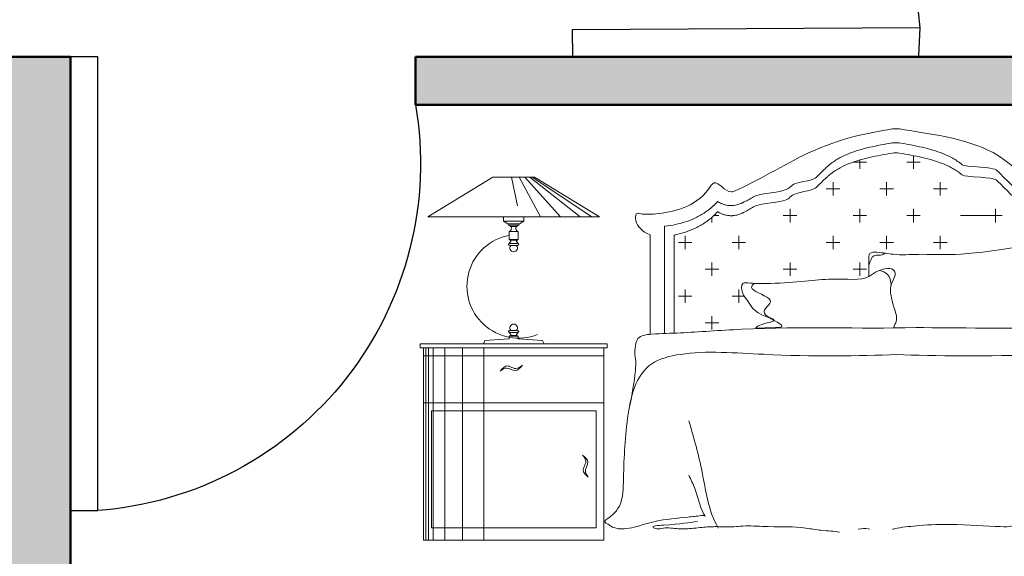
# Model space of a CAD drawing. Units: inches. Extents: x 1771 to 3025, y 319 to 889.
# Tile 16 of 35: x 2402 to 2505, y 564 to 621. Entities that reach past the tile are written whole.
import ezdxf

# ---------------------------------------------------------------- set-up
doc = ezdxf.new("R2010")
doc.units = ezdxf.units.IN
doc.header["$MEASUREMENT"] = 0
for name, color, linetype, lineweight in [('A-DOOR', 4, 'Continuous', 25), ('A-FURN', 8, 'Continuous', 18), ('A-WALL', 7, 'Continuous', 50), ('A-WALL-PATT', 254, 'Continuous', 13)]:
    doc.layers.add(name, color=color, linetype=linetype, lineweight=lineweight)

# ---------------------------------------------------------------- blocks, each defined once
blk = doc.blocks.new('A$C3908634B')
at = {"ltscale": 5}
for p, q in [((1200.2, 1046.3), (1218.1, 1046.3)), ((1176, 731), (1176, 731.7))]:
    blk.add_line(p, q, dxfattribs=at)
for p, q in [((1253.9, 945.1), (1253.9, 978.5)), ((1100.9, 962.2), (1134.6, 962.2)), ((1117.6, 945.1), (1117.6, 967.5)), ((1236.9, 962.2), (1271, 962.2)), ((184.3, 923.4), (19, 823.1)), ((237.5, 923.4), (184.3, 923.4)), ((190.2, 923.4), (237.5, 923.4)), ((231.9, 923.4), (247.3, 851.1)), ((284.7, 923.4), (237.5, 923.4)), ((237.5, 923.4), (290.6, 923.4)), ((251.7, 923.4), (305.7, 823.1)), ((266, 923.4), (356.4, 823.1)), ((278.7, 923.4), (406.8, 823.1)), ((284.7, 923.4), (436.3, 823.1)), ((290.6, 923.4), (456, 823.1)), ((1049.4, 876.9), (1049.4, 911)), ((1185.7, 876.9), (1185.7, 911)), ((1322.1, 876.9), (1322.1, 911)), ((2198.9, 923.4), (2033.5, 823.1)), ((2204.8, 923.4), (2053.3, 823.1)), ((2210.8, 923.4), (2082.7, 823.1)), ((2223.5, 923.4), (2133.1, 823.1)), ((2237.8, 923.4), (2183.8, 823.1)), ((2252, 923.4), (2198.9, 923.4)), ((2204.8, 923.4), (2252, 923.4)), ((2257.6, 923.4), (2242.2, 851.1)), ((2299.3, 923.4), (2252, 923.4)), ((2252, 923.4), (2305.2, 923.4)), ((2305.2, 923.4), (2470.5, 823.1)), ((1032.3, 894), (1066.4, 894)), ((1168.7, 894), (1202.8, 894)), ((1305.1, 894), (1339.1, 894)), ((940, 808.8), (940, 842.9)), ((1117.6, 808.8), (1117.6, 842.9)), ((1253.9, 808.8), (1253.9, 842.9)), ((1462.5, 808.8), (1462.5, 842.9)), ((237.5, 823.1), (19, 823.1)), ((212, 823.1), (212, 811.7)), ((212, 811.7), (223, 805.4)), ((212, 811.7), (237.5, 811.7)), ((223, 805.4), (224.6, 801.4)), ((223, 805.4), (237.5, 805.4)), ((250.4, 801.4), (224.6, 801.4)), ((226.9, 801.4), (228.3, 798.3)), ((237.5, 823.1), (456, 823.1)), ((263, 811.7), (237.5, 811.7)), ((252, 805.4), (237.5, 805.4)), ((248.1, 801.4), (246.7, 798.3)), ((252, 805.4), (250.4, 801.4)), ((263, 811.7), (252, 805.4)), ((263, 823.1), (263, 811.7)), ((741.7, 808.8), (741.7, 821.7)), ((746.2, 825.8), (758.8, 825.8)), ((922.9, 825.8), (957, 825.8)), ((1100.5, 825.8), (1134.6, 825.8)), ((1236.9, 825.8), (1271, 825.8)), ((1373.2, 825.8), (1479.5, 825.8)), ((1681.3, 808.8), (1681.3, 825.6)), ((2252, 823.1), (2033.5, 823.1)), ((2226.5, 823.1), (2226.5, 811.7)), ((2226.5, 811.7), (2237.6, 805.4)), ((2226.5, 811.7), (2252, 811.7)), ((2237.6, 805.4), (2239.1, 801.4)), ((2237.6, 805.4), (2252, 805.4)), ((2239.1, 801.4), (2264.9, 801.4)), ((2241.4, 801.4), (2242.8, 798.3)), ((2252, 823.1), (2470.5, 823.1)), ((2277.6, 811.7), (2252, 811.7)), ((2266.5, 805.4), (2252, 805.4)), ((2262.6, 801.4), (2261.2, 798.3)), ((2266.5, 805.4), (2264.9, 801.4)), ((2277.6, 811.7), (2266.5, 805.4)), ((2277.6, 823.1), (2277.6, 811.7)), ((227.8, 786.4), (226.2, 785.6)), ((226.2, 785.6), (226.2, 765)), ((226.2, 785.6), (248.8, 785.6)), ((230.2, 788), (227.8, 786.4)), ((228.3, 798.3), (237.5, 798.3)), ((228.3, 798.3), (231.3, 797.6)), ((231.1, 790.5), (230.2, 788)), ((231.5, 791.1), (231.1, 790.5)), ((231.3, 797.6), (232, 794.9)), ((231.6, 792.6), (231.5, 791.9)), ((231.5, 791.9), (231.5, 791.1)), ((231.9, 793.9), (231.6, 792.6)), ((232, 794.9), (231.9, 793.9)), ((246.7, 798.3), (237.5, 798.3)), ((243.7, 797.6), (243, 794.9)), ((243, 794.9), (243.1, 793.9)), ((243.1, 793.9), (243.4, 792.6)), ((243.4, 792.6), (243.4, 791.9)), ((243.4, 791.9), (243.4, 791.1)), ((243.4, 791.1), (243.9, 790.5)), ((246.7, 798.3), (243.7, 797.6)), ((243.9, 790.5), (244.8, 788)), ((244.8, 788), (247.2, 786.4)), ((247.2, 786.4), (248.8, 785.6)), ((248.8, 785.6), (248.8, 765)), ((621.3, 798.8), (621.3, 526)), ((645.8, 776.5), (645.8, 527)), ((1824, 776.5), (1824, 527.2)), ((1848.6, 798.8), (1848.6, 526.2)), ((2242.3, 786.4), (2240.7, 785.6)), ((2240.7, 785.6), (2240.7, 765)), ((2263.3, 785.6), (2240.7, 785.6)), ((2244.7, 788), (2242.3, 786.4)), ((2242.8, 798.3), (2245.8, 797.6)), ((2242.8, 798.3), (2252, 798.3)), ((2245.6, 790.5), (2244.7, 788)), ((2246.1, 791.1), (2245.6, 790.5)), ((2245.8, 797.6), (2246.5, 794.9)), ((2246.4, 793.9), (2246.1, 792.6)), ((2246.1, 792.6), (2246.1, 791.9)), ((2246.1, 791.9), (2246.1, 791.1)), ((2246.5, 794.9), (2246.4, 793.9)), ((2261.2, 798.3), (2252, 798.3)), ((2258.2, 797.6), (2257.6, 794.9)), ((2257.6, 794.9), (2257.6, 793.9)), ((2257.6, 793.9), (2257.9, 792.6)), ((2257.9, 792.6), (2258, 791.9)), ((2258, 791.9), (2258, 791.1)), ((2258, 791.1), (2258.4, 790.5)), ((2261.2, 798.3), (2258.2, 797.6)), ((2258.4, 790.5), (2259.4, 788)), ((2259.4, 788), (2261.7, 786.4)), ((2261.7, 786.4), (2263.3, 785.6)), ((2263.3, 785.6), (2263.3, 765)), ((224.8, 753.5), (224.7, 752.9)), ((224.7, 752.9), (224.8, 752.1)), ((225.3, 753.9), (224.8, 753.5)), ((224.8, 752.1), (225.2, 751.4)), ((225.2, 751.4), (225.6, 750.9)), ((225.7, 754.3), (225.3, 753.9)), ((225.6, 750.9), (228.1, 750.2)), ((226.3, 754.6), (225.7, 754.3)), ((226.2, 765), (227.6, 764.2)), ((226.2, 765), (237.5, 765)), ((227, 754.7), (226.3, 754.6)), ((227.9, 754.7), (227, 754.7)), ((227.4, 757.9), (227.1, 757.2)), ((227.1, 757.2), (227.3, 756.6)), ((227.3, 756.6), (227.8, 755.9)), ((227.7, 758.5), (227.4, 757.9)), ((227.6, 764.2), (228.5, 763.3)), ((228.6, 758.7), (227.7, 758.5)), ((227.8, 755.9), (228.9, 755.2)), ((228.9, 755.2), (227.9, 754.7)), ((228.5, 763.3), (229.4, 762.5)), ((228.5, 763.3), (237.5, 763.3)), ((229.4, 759.1), (228.6, 758.7)), ((228.9, 755.2), (237.5, 755.2)), ((229.4, 762.5), (230, 761.4)), ((229.8, 759.5), (229.4, 759.1)), ((230.1, 760.2), (229.8, 759.5)), ((230, 761.4), (230.1, 760.2)), ((248.8, 765), (237.5, 765)), ((246.5, 763.3), (237.5, 763.3)), ((246.1, 755.2), (237.5, 755.2)), ((245, 761.4), (244.9, 760.2)), ((244.9, 760.2), (245.2, 759.5)), ((245.6, 762.5), (245, 761.4)), ((245.2, 759.5), (245.6, 759.1)), ((246.5, 763.3), (245.6, 762.5)), ((245.6, 759.1), (246.4, 758.7)), ((247.2, 755.9), (246.1, 755.2)), ((246.1, 755.2), (247.1, 754.7)), ((246.4, 758.7), (247.3, 758.5)), ((247.4, 764.2), (246.5, 763.3)), ((249.4, 750.9), (246.9, 750.2)), ((247.1, 754.7), (248, 754.7)), ((247.7, 756.6), (247.2, 755.9)), ((247.3, 758.5), (247.6, 757.9)), ((248.8, 765), (247.4, 764.2)), ((247.6, 757.9), (247.9, 757.2)), ((247.9, 757.2), (247.7, 756.6)), ((248, 754.7), (248.7, 754.6)), ((248.7, 754.6), (249.3, 754.3)), ((249.3, 754.3), (249.7, 753.9)), ((249.8, 751.4), (249.4, 750.9)), ((249.7, 753.9), (250.2, 753.5)), ((250.2, 752.1), (249.8, 751.4)), ((250.2, 753.5), (250.3, 752.9)), ((250.3, 752.9), (250.2, 752.1)), ((656.5, 757.6), (690.6, 757.6)), ((673.5, 740.6), (673.5, 774.7)), ((792.9, 757.6), (827, 757.6)), ((809.9, 740.6), (809.9, 774.7)), ((1032.3, 757.6), (1066.4, 757.6)), ((1049.4, 740.6), (1049.4, 774.7)), ((1168.7, 757.6), (1202.8, 757.6)), ((1185.7, 740.6), (1185.7, 774.7)), ((1305.1, 757.6), (1339.1, 757.6)), ((1322.1, 740.6), (1322.1, 774.7)), ((1513.6, 757.6), (1547.7, 757.6)), ((1530.6, 751.3), (1530.6, 774.7)), ((1732.4, 757.6), (1766.5, 757.6)), ((1749.5, 740.6), (1749.5, 774.7)), ((2239.4, 753.5), (2239.2, 752.9)), ((2239.2, 752.9), (2239.3, 752.1)), ((2239.3, 752.1), (2239.7, 751.4)), ((2239.9, 753.9), (2239.4, 753.5)), ((2239.7, 751.4), (2240.2, 750.9)), ((2240.3, 754.3), (2239.9, 753.9)), ((2240.2, 750.9), (2242.6, 750.2)), ((2240.8, 754.6), (2240.3, 754.3)), ((2240.7, 765), (2242.1, 764.2)), ((2240.7, 765), (2252, 765)), ((2241.5, 754.7), (2240.8, 754.6)), ((2242.4, 754.7), (2241.5, 754.7)), ((2241.9, 757.9), (2241.7, 757.2)), ((2241.7, 757.2), (2241.8, 756.6)), ((2241.8, 756.6), (2242.3, 755.9)), ((2242.2, 758.5), (2241.9, 757.9)), ((2242.1, 764.2), (2243, 763.3)), ((2243.1, 758.7), (2242.2, 758.5)), ((2242.3, 755.9), (2243.4, 755.2)), ((2243.4, 755.2), (2242.4, 754.7)), ((2243, 763.3), (2243.9, 762.5)), ((2243, 763.3), (2252, 763.3)), ((2243.9, 759.1), (2243.1, 758.7)), ((2243.4, 755.2), (2252, 755.2)), ((2243.9, 762.5), (2244.6, 761.4)), ((2244.3, 759.5), (2243.9, 759.1)), ((2244.6, 760.2), (2244.3, 759.5)), ((2244.6, 761.4), (2244.6, 760.2)), ((2263.3, 765), (2252, 765)), ((2261.1, 763.3), (2252, 763.3)), ((2260.7, 755.2), (2252, 755.2)), ((2259.5, 761.4), (2259.4, 760.2)), ((2259.4, 760.2), (2259.7, 759.5)), ((2260.1, 762.5), (2259.5, 761.4)), ((2259.7, 759.5), (2260.1, 759.1)), ((2261.1, 763.3), (2260.1, 762.5)), ((2260.1, 759.1), (2260.9, 758.7)), ((2261.8, 755.9), (2260.7, 755.2)), ((2260.7, 755.2), (2261.6, 754.7)), ((2260.9, 758.7), (2261.8, 758.5)), ((2261.9, 764.2), (2261.1, 763.3)), ((2263.9, 750.9), (2261.5, 750.2)), ((2261.6, 754.7), (2262.5, 754.7)), ((2261.8, 758.5), (2262.2, 757.9)), ((2262.2, 756.6), (2261.8, 755.9)), ((2263.3, 765), (2261.9, 764.2)), ((2262.2, 757.9), (2262.4, 757.2)), ((2262.4, 757.2), (2262.2, 756.6)), ((2262.5, 754.7), (2263.2, 754.6)), ((2263.2, 754.6), (2263.8, 754.3)), ((2263.8, 754.3), (2264.2, 753.9)), ((2264.3, 751.4), (2263.9, 750.9)), ((2264.2, 753.9), (2264.7, 753.5)), ((2264.7, 752.1), (2264.3, 751.4)), ((2264.7, 753.5), (2264.8, 752.9)), ((2264.8, 752.9), (2264.7, 752.1)), ((228.1, 750.2), (229.9, 750)), ((229.9, 750), (232.4, 750.2)), ((232.4, 750.2), (237.5, 750.2)), ((242.6, 750.2), (237.5, 750.2)), ((245.1, 750), (242.6, 750.2)), ((246.9, 750.2), (245.1, 750)), ((2242.6, 750.2), (2244.4, 750)), ((2244.4, 750), (2246.9, 750.2)), ((2246.9, 750.2), (2252, 750.2)), ((2257.1, 750.2), (2252, 750.2)), ((2259.6, 750), (2257.1, 750.2)), ((2261.5, 750.2), (2259.6, 750)), ((741.7, 672.4), (741.7, 706.5)), ((940, 672.4), (940, 706.5)), ((1117.6, 672.4), (1117.6, 706.5)), ((1681.3, 672.4), (1681.3, 706.5)), ((1817.7, 672.4), (1817.7, 706.5)), ((724.7, 689.4), (758.8, 689.4)), ((922.9, 689.4), (957, 689.4)), ((1100.5, 689.4), (1134.6, 689.4)), ((1664.3, 689.4), (1698.3, 689.4)), ((1800.6, 689.4), (1824, 689.4)), ((673.5, 604.2), (673.5, 638.3)), ((809.9, 604.2), (809.9, 638.3)), ((1749.5, 604.2), (1749.5, 638.3)), ((656.5, 621.3), (690.6, 621.3)), ((792.9, 621.3), (823.2, 621.3)), ((1732.4, 621.3), (1766.5, 621.3)), ((724.7, 553.1), (758.8, 553.1)), ((741.7, 536), (741.7, 570.1)), ((1664.3, 553.1), (1698.3, 553.1)), ((1681.3, 536), (1681.3, 570.1)), ((1800.6, 553.1), (1824, 553.1)), ((1817.7, 536), (1817.7, 570.1)), ((224.7, 530.9), (224.8, 531.7)), ((224.8, 530.3), (224.7, 530.9)), ((224.8, 531.7), (225.2, 532.4)), ((225.3, 529.9), (224.8, 530.3)), ((225.2, 532.4), (225.6, 532.9)), ((225.7, 529.5), (225.3, 529.9)), ((225.6, 532.9), (228.1, 533.6)), ((226.3, 529.2), (225.7, 529.5)), ((227, 529.1), (226.3, 529.2)), ((227.9, 529.1), (227, 529.1)), ((227.1, 526.6), (227.3, 527.2)), ((227.4, 525.9), (227.1, 526.6)), ((227.3, 527.2), (227.8, 527.9)), ((227.7, 525.3), (227.4, 525.9)), ((227.8, 527.9), (228.9, 528.6)), ((228.9, 528.6), (227.9, 529.1)), ((228.1, 533.6), (229.9, 533.8)), ((228.9, 528.6), (237.5, 528.6)), ((230.3, 533.8), (237.5, 533.6)), ((242.6, 533.6), (237.5, 533.6)), ((246.1, 528.6), (237.5, 528.6)), ((245.1, 533.8), (242.6, 533.6)), ((246.9, 533.6), (245.1, 533.8)), ((246.1, 528.6), (247.1, 529.1)), ((247.2, 527.9), (246.1, 528.6)), ((249.4, 532.9), (246.9, 533.6)), ((247.1, 529.1), (248, 529.1)), ((247.7, 527.2), (247.2, 527.9)), ((247.3, 525.3), (247.6, 525.9)), ((247.6, 525.9), (247.9, 526.6)), ((247.9, 526.6), (247.7, 527.2)), ((248, 529.1), (248.7, 529.2)), ((248.7, 529.2), (249.3, 529.5)), ((249.3, 529.5), (249.7, 529.9)), ((249.8, 532.4), (249.4, 532.9)), ((249.7, 529.9), (250.2, 530.3)), ((250.2, 531.7), (249.8, 532.4)), ((250.3, 530.9), (250.2, 531.7)), ((250.2, 530.3), (250.3, 530.9)), ((2239.2, 530.9), (2239.3, 531.7)), ((2239.4, 530.3), (2239.2, 530.9)), ((2239.3, 531.7), (2239.7, 532.4)), ((2239.9, 529.9), (2239.4, 530.3)), ((2239.7, 532.4), (2240.2, 532.9)), ((2240.3, 529.5), (2239.9, 529.9)), ((2240.2, 532.9), (2242.6, 533.6)), ((2240.8, 529.2), (2240.3, 529.5)), ((2241.5, 529.1), (2240.8, 529.2)), ((2242.4, 529.1), (2241.5, 529.1)), ((2241.7, 526.6), (2241.8, 527.2)), ((2241.9, 525.9), (2241.7, 526.6)), ((2241.8, 527.2), (2242.3, 527.9)), ((2242.2, 525.3), (2241.9, 525.9)), ((2242.3, 527.9), (2243.4, 528.6)), ((2243.4, 528.6), (2242.4, 529.1)), ((2242.6, 533.6), (2244.4, 533.8)), ((2243.4, 528.6), (2252, 528.6)), ((2244.4, 533.8), (2246.9, 533.6)), ((2246.9, 533.6), (2252, 533.6)), ((2259.2, 533.8), (2252, 533.6)), ((2260.7, 528.6), (2252, 528.6)), ((2261.5, 533.6), (2259.6, 533.8)), ((2260.7, 528.6), (2261.6, 529.1)), ((2261.8, 527.9), (2260.7, 528.6)), ((2263.9, 532.9), (2261.5, 533.6)), ((2261.6, 529.1), (2262.5, 529.1)), ((2262.2, 527.2), (2261.8, 527.9)), ((2261.8, 525.3), (2262.2, 525.9)), ((2262.4, 526.6), (2262.2, 527.2)), ((2262.2, 525.9), (2262.4, 526.6)), ((2262.5, 529.1), (2263.2, 529.2)), ((2263.2, 529.2), (2263.8, 529.5)), ((2263.8, 529.5), (2264.2, 529.9)), ((2264.3, 532.4), (2263.9, 532.9)), ((2264.2, 529.9), (2264.7, 530.3)), ((2264.7, 531.7), (2264.3, 532.4)), ((2264.8, 530.9), (2264.7, 531.7)), ((2264.7, 530.3), (2264.8, 530.9)), ((164, 507.9), (161.1, 499.5)), ((164, 507.9), (226.2, 512.1)), ((226.2, 518.8), (227.6, 519.6)), ((226.2, 512.1), (226.2, 518.8)), ((226.2, 518.8), (237.5, 518.8)), ((227.6, 519.6), (228.5, 520.5)), ((228.6, 525.1), (227.7, 525.3)), ((228.5, 520.5), (229.4, 521.3)), ((229.4, 524.7), (228.6, 525.1)), ((229.8, 524.3), (229.4, 524.7)), ((229.4, 521.3), (230, 522.4)), ((229.4, 521.3), (237.5, 521.3)), ((230.1, 523.6), (229.8, 524.3)), ((230, 522.4), (230.1, 523.6)), ((245.6, 521.3), (237.5, 521.3)), ((248.8, 518.8), (237.5, 518.8)), ((244.9, 523.6), (245.2, 524.3)), ((245, 522.4), (244.9, 523.6)), ((245.6, 521.3), (245, 522.4)), ((245.2, 524.3), (245.6, 524.7)), ((245.6, 524.7), (246.4, 525.1)), ((246.5, 520.5), (245.6, 521.3)), ((246.4, 525.1), (247.3, 525.3)), ((247.4, 519.6), (246.5, 520.5)), ((248.8, 518.8), (247.4, 519.6)), ((248.8, 512.1), (248.8, 518.8)), ((311, 507.9), (248.8, 512.1)), ((311, 507.9), (315.3, 499.5)), ((2178.5, 507.9), (2174.2, 499.5)), ((2178.5, 507.9), (2240.7, 512.1)), ((2240.7, 518.8), (2242.1, 519.6)), ((2240.7, 512.1), (2240.7, 518.8)), ((2240.7, 518.8), (2252, 518.8)), ((2242.1, 519.6), (2243, 520.5)), ((2243.1, 525.1), (2242.2, 525.3)), ((2243, 520.5), (2243.9, 521.3)), ((2243.9, 524.7), (2243.1, 525.1)), ((2244.3, 524.3), (2243.9, 524.7)), ((2243.9, 521.3), (2244.6, 522.4)), ((2243.9, 521.3), (2252, 521.3)), ((2244.6, 523.6), (2244.3, 524.3)), ((2244.6, 522.4), (2244.6, 523.6)), ((2260.1, 521.3), (2252, 521.3)), ((2263.3, 518.8), (2252, 518.8)), ((2259.4, 523.6), (2259.7, 524.3)), ((2259.5, 522.4), (2259.4, 523.6)), ((2260.1, 521.3), (2259.5, 522.4)), ((2259.7, 524.3), (2260.1, 524.7)), ((2260.1, 524.7), (2260.9, 525.1)), ((2261.1, 520.5), (2260.1, 521.3)), ((2260.9, 525.1), (2261.8, 525.3)), ((2261.9, 519.6), (2261.1, 520.5)), ((2263.3, 518.8), (2261.9, 519.6)), ((2263.3, 512.1), (2263.3, 518.8)), ((2325.5, 507.9), (2263.3, 512.1)), ((2325.5, 507.9), (2328.4, 499.5)), ((475, 499.5), (0, 499.5)), ((0, 499.5), (0, 489.5)), ((475, 489.5), (0, 489.5)), ((8.7, 489.5), (8.7, 0)), ((14.1, 488.6), (14.1, 0)), ((21.3, 488.6), (21.3, 0)), ((33, 488.6), (33, 0)), ((62.7, 488.6), (62.7, 0)), ((107.6, 488.6), (107.6, 0)), ((161.1, 499.5), (237.5, 499.5)), ((161.6, 488.6), (161.6, 0)), ((315.3, 499.5), (237.5, 499.5)), ((467.1, 0), (467.1, 489.5)), ((475, 499.5), (475, 489.5)), ((2014.5, 499.5), (2489.5, 499.5)), ((2014.5, 499.5), (2014.5, 489.5)), ((2014.5, 489.5), (2489.5, 489.5)), ((2022.4, 0), (2022.4, 489.5)), ((2174.2, 499.5), (2252, 499.5)), ((2328.4, 499.5), (2252, 499.5)), ((2327.9, 488.6), (2327.9, 0)), ((2381.9, 488.6), (2381.9, 0)), ((2426.8, 488.6), (2426.8, 0)), ((2456.5, 488.6), (2456.5, 0)), ((2468.2, 488.6), (2468.2, 0)), ((2475.4, 488.6), (2475.4, 0)), ((2480.8, 489.5), (2480.8, 0)), ((2489.5, 499.5), (2489.5, 489.5)), ((467.1, 469.5), (8.7, 469.5)), ((2022.4, 469.5), (2480.8, 469.5)), ((467.1, 349.5), (8.7, 349.5)), ((28.7, 329.5), (28.7, 31.6)), ((447.1, 329.5), (28.7, 329.5)), ((447.1, 31.6), (447.1, 329.5)), ((2022.4, 349.5), (2480.8, 349.5)), ((2042.4, 329.5), (2460.8, 329.5)), ((2042.4, 31.6), (2042.4, 329.5)), ((2460.8, 329.5), (2460.8, 31.6)), ((467.1, 281.6), (467.1, 301.6)), ((2022.4, 281.6), (2022.4, 301.6)), ((28.7, 31.6), (447.1, 31.6)), ((2460.8, 31.6), (2042.4, 31.6)), ((8.7, 0), (467.1, 0)), ((2022.4, 0), (2480.8, 0))]:
    blk.add_line(p, q)
at = {"ltscale": 20}
for p, q in [((584.4, 776.7), (584.4, 523.7)), ((1885.4, 776.7), (1885.4, 524))]:
    blk.add_line(p, q, dxfattribs=at)
for centre, radius, start, end in [((1209.1, 956.2), 55.2, 80.5605, 99.4395), ((1209.1, 930.3), 55.2, 80.5605, 99.4395), ((250.5, 646.2), 131.8, 100.6234, 291.2), ((2239, 646.2), 131.8, 248.8, 79.3766), ((237.5, 743.5), 9.69, 137.7341, 270), ((237.5, 743.5), 9.69, 270, 42.2659), ((2252, 743.5), 9.69, 137.7341, 270), ((2252, 743.5), 9.69, 270, 42.2659), ((237.5, 540.3), 9.69, 90, 222.2659), ((237.5, 540.3), 9.69, 317.7341, 90), ((2252, 540.3), 9.69, 90, 222.2659), ((2252, 540.3), 9.69, 317.7341, 90)]:
    blk.add_arc(centre, radius, start, end)
for points in [[(584.4, 776.7), (563.9, 786.2), (546, 802.1), (547.3, 834.8), (564.5, 828.3), (620.6, 830.4), (706.4, 847.2), (752.1, 924.2), (778.1, 880.4), (846.1, 907.1), (1017.7, 1014.1), (1134.5, 1035.5), (1200.2, 1046.3)], [(1885.4, 776.7), (1905.9, 786.2), (1923.9, 802.1), (1922.5, 834.8), (1905.3, 828.3), (1849.2, 830.4), (1763.4, 847.2), (1717.7, 924.2), (1691.7, 880.4), (1541.2, 907.1), (1472.8, 1014.1), (1283.8, 1035.5), (1218.1, 1046.3)]]:
    blk.add_open_spline(points, degree=3, knots=[12.417853, 12.417853, 12.417853, 12.417853, 68.394536, 90.665986, 114.156853, 157.554067, 281.869614, 298.858744, 338.737111, 347.060176, 470.423438, 625.498764, 625.498764, 625.498764, 625.498764], dxfattribs=at)
for points, knots in [([(756.1, 861.8), (756.9, 861.3), (757.6, 860.9), (759.9, 859.6), (761.6, 858.7), (765.5, 856.8), (767.8, 855.8), (772.7, 854.1), (775.4, 853.3), (780.8, 852.2), (783.3, 851.8), (787.1, 851.6), (788.2, 851.5), (789.9, 851.5), (790.6, 851.5), (791.9, 851.5), (792.5, 851.5), (793.6, 851.6), (794.1, 851.6), (795.8, 851.8), (796.8, 851.9), (800.3, 852.3), (802.5, 852.8), (806.5, 853.8), (808.3, 854.3), (811.5, 855.4), (812.9, 855.9), (815.3, 856.9), (816.4, 857.4), (817.6, 857.9), (817.8, 858), (818.4, 858.2), (818.7, 858.4), (819.5, 858.7), (820, 859), (821.6, 859.7), (822.7, 860.2), (825.8, 861.7), (827.9, 862.8), (834, 866), (837.9, 868.3), (848.5, 874.9), (854.9, 879.4), (928.8, 888.8), (934.4, 893.5), (945, 903.2), (950, 908), (1000.9, 917.4), (1005.5, 922.1), (1014.4, 931), (1018.7, 935.3), (1027, 943.5), (1031.1, 947.3), (1036.9, 952.4), (1038.8, 954), (1042, 956.7), (1043.5, 957.9), (1045.8, 959.7), (1046.7, 960.3), (1048.5, 961.7), (1049.4, 962.3), (1052.1, 964.2), (1054, 965.5), (1059.7, 969.2), (1063.6, 971.5), (1074.8, 977.5), (1082.2, 980.9), (1098, 987.2), (1106.3, 990), (1123.7, 995.2), (1132.8, 997.5), (1151.5, 1001.8), (1161.1, 1003.8), (1180.5, 1007.4), (1190.2, 1009), (1200.1, 1010.7)], [328.6705, 328.6705, 328.6705, 328.6705, 329.609368, 329.609368, 331.487103, 331.487103, 333.620342, 333.620342, 335.753581, 335.753581, 337.507866, 337.507866, 338.182373, 338.182373, 338.607397, 338.607397, 338.959312, 338.959312, 339.311227, 339.311227, 340.015058, 340.015058, 341.722742, 341.722742, 343.430427, 343.430427, 345.138111, 345.138111, 346.845796, 346.845796, 347.37881, 347.37881, 347.911824, 347.911824, 348.977853, 348.977853, 351.109909, 351.109909, 355.374023, 355.374023, 363.902249, 363.902249, 379.258481, 379.258481, 394.614712, 394.614712, 409.970944, 409.970944, 425.327175, 425.327175, 440.683406, 440.683406, 456.039638, 456.039638, 463.285514, 463.285514, 469.01116, 469.01116, 472.593, 472.593, 476.17484, 476.17484, 483.338521, 483.338521, 497.665882, 497.665882, 522.309302, 522.309302, 546.952723, 546.952723, 571.596143, 571.596143, 596.239564, 596.239564, 619.876409, 619.876409, 619.876409, 619.876409]), ([(1713.7, 861.8), (1713, 861.3), (1712.2, 860.9), (1709.9, 859.6), (1708.2, 858.7), (1704.3, 856.8), (1702.1, 855.8), (1697.1, 854.1), (1694.4, 853.3), (1689.1, 852.2), (1686.5, 851.8), (1682.7, 851.6), (1681.7, 851.5), (1679.9, 851.5), (1679.2, 851.5), (1678, 851.5), (1677.4, 851.5), (1676.2, 851.6), (1675.7, 851.6), (1674.1, 851.8), (1673, 851.9), (1669.5, 852.3), (1667.3, 852.8), (1663.3, 853.8), (1661.5, 854.3), (1658.4, 855.4), (1657, 855.9), (1654.5, 856.9), (1653.4, 857.4), (1652.2, 857.9), (1652, 858), (1651.4, 858.2), (1651.2, 858.4), (1650.4, 858.7), (1649.8, 859), (1648.2, 859.7), (1647.1, 860.2), (1644, 861.7), (1641.9, 862.8), (1553.3, 866), (1549.4, 868.3), (1538.8, 874.9), (1532.4, 879.4), (1520.4, 888.8), (1514.8, 893.5), (1504.2, 903.2), (1499.2, 908), (1489.5, 917.4), (1484.9, 922.1), (1476.1, 931), (1471.8, 935.3), (1463.4, 943.5), (1459.4, 947.3), (1381.4, 952.4), (1379.5, 954), (1376.2, 956.7), (1374.8, 957.9), (1372.5, 959.7), (1371.6, 960.3), (1369.8, 961.7), (1368.9, 962.3), (1366.2, 964.2), (1364.3, 965.5), (1358.6, 969.2), (1354.6, 971.5), (1343.5, 977.5), (1336, 980.9), (1320.2, 987.2), (1311.9, 990), (1294.6, 995.2), (1285.5, 997.5), (1266.8, 1001.8), (1257.2, 1003.8), (1237.8, 1007.4), (1228.1, 1009), (1218.2, 1010.7)], [328.6705, 328.6705, 328.6705, 328.6705, 329.609368, 329.609368, 331.487103, 331.487103, 333.620342, 333.620342, 335.753581, 335.753581, 337.507866, 337.507866, 338.182373, 338.182373, 338.607397, 338.607397, 338.959312, 338.959312, 339.311227, 339.311227, 340.015058, 340.015058, 341.722742, 341.722742, 343.430427, 343.430427, 345.138111, 345.138111, 346.845796, 346.845796, 347.37881, 347.37881, 347.911824, 347.911824, 348.977853, 348.977853, 351.109909, 351.109909, 355.374023, 355.374023, 363.902249, 363.902249, 379.258481, 379.258481, 394.614712, 394.614712, 409.970943, 409.970943, 425.327175, 425.327175, 440.683406, 440.683406, 456.039637, 456.039637, 463.285514, 463.285514, 469.011154, 469.011154, 472.592992, 472.592992, 476.17483, 476.17483, 483.338506, 483.338506, 497.665857, 497.665857, 522.309275, 522.309275, 546.952693, 546.952693, 571.59611, 571.59611, 596.239528, 596.239528, 619.876409, 619.876409, 619.876409, 619.876409]), ([(756.1, 835.9), (756.9, 835.5), (757.6, 835), (759.9, 833.7), (761.6, 832.8), (765.5, 830.9), (767.8, 830), (772.7, 828.2), (775.4, 827.5), (780.8, 826.3), (783.3, 826), (787.1, 825.7), (788.2, 825.7), (789.9, 825.6), (790.6, 825.6), (791.9, 825.6), (792.5, 825.7), (793.6, 825.7), (794.1, 825.8), (795.8, 825.9), (796.8, 826), (800.3, 826.5), (802.5, 826.9), (806.5, 827.9), (808.3, 828.5), (811.5, 829.5), (812.9, 830.1), (815.3, 831), (816.4, 831.5), (817.6, 832), (817.8, 832.1), (818.4, 832.4), (818.7, 832.5), (819.5, 832.9), (820, 833.1), (821.6, 833.8), (822.7, 834.3), (825.8, 835.9), (827.9, 836.9), (834, 840.2), (837.9, 842.4), (848.5, 849), (854.9, 853.6), (928.8, 862.9), (934.4, 867.7), (945, 877.3), (950, 882.1), (1000.9, 891.6), (1005.5, 896.2), (1014.4, 905.2), (1018.7, 909.5), (1027, 917.6), (1031.1, 921.4), (1036.9, 926.6), (1038.8, 928.2), (1042, 930.9), (1043.5, 932), (1045.8, 933.8), (1046.7, 934.5), (1048.5, 935.8), (1049.4, 936.4), (1052.1, 938.4), (1054, 939.6), (1059.7, 943.3), (1063.6, 945.6), (1074.8, 951.6), (1082.2, 955), (1098, 961.3), (1106.3, 964.2), (1123.7, 969.3), (1132.8, 971.6), (1151.5, 975.9), (1161.1, 977.9), (1180.5, 981.5), (1190.2, 983.2), (1200.1, 984.8)], [328.6705, 328.6705, 328.6705, 328.6705, 329.609368, 329.609368, 331.487103, 331.487103, 333.620342, 333.620342, 335.753581, 335.753581, 337.507866, 337.507866, 338.182373, 338.182373, 338.607397, 338.607397, 338.959312, 338.959312, 339.311227, 339.311227, 340.015058, 340.015058, 341.722742, 341.722742, 343.430427, 343.430427, 345.138111, 345.138111, 346.845796, 346.845796, 347.37881, 347.37881, 347.911824, 347.911824, 348.977853, 348.977853, 351.109909, 351.109909, 355.374023, 355.374023, 363.902249, 363.902249, 379.258481, 379.258481, 394.614712, 394.614712, 409.970944, 409.970944, 425.327175, 425.327175, 440.683406, 440.683406, 456.039638, 456.039638, 463.285514, 463.285514, 469.01116, 469.01116, 472.593, 472.593, 476.17484, 476.17484, 483.338521, 483.338521, 497.665882, 497.665882, 522.309302, 522.309302, 546.952723, 546.952723, 571.596143, 571.596143, 596.239564, 596.239564, 619.876409, 619.876409, 619.876409, 619.876409]), ([(1713.7, 835.9), (1713, 835.5), (1712.2, 835), (1709.9, 833.7), (1708.2, 832.8), (1704.3, 830.9), (1702.1, 830), (1697.1, 828.2), (1694.4, 827.5), (1689.1, 826.3), (1686.5, 826), (1682.7, 825.7), (1681.7, 825.7), (1679.9, 825.6), (1679.2, 825.6), (1678, 825.6), (1677.4, 825.7), (1676.2, 825.7), (1675.7, 825.8), (1674.1, 825.9), (1673, 826), (1669.5, 826.5), (1667.3, 826.9), (1663.3, 827.9), (1661.5, 828.5), (1658.4, 829.5), (1657, 830.1), (1654.5, 831), (1653.4, 831.5), (1652.2, 832), (1652, 832.1), (1651.4, 832.4), (1651.2, 832.5), (1650.4, 832.9), (1649.8, 833.1), (1648.2, 833.8), (1647.1, 834.3), (1644, 835.9), (1641.9, 836.9), (1553.3, 840.2), (1549.4, 842.4), (1538.8, 849), (1532.4, 853.6), (1520.4, 862.9), (1514.8, 867.7), (1504.2, 877.3), (1499.2, 882.1), (1489.5, 891.6), (1484.9, 896.2), (1476.1, 905.2), (1471.8, 909.5), (1463.4, 917.6), (1459.4, 921.4), (1381.4, 926.6), (1379.5, 928.2), (1376.2, 930.9), (1374.8, 932), (1372.5, 933.8), (1371.6, 934.5), (1369.8, 935.8), (1368.9, 936.4), (1366.2, 938.4), (1364.3, 939.6), (1358.6, 943.3), (1354.6, 945.6), (1343.5, 951.6), (1336, 955), (1320.2, 961.3), (1311.9, 964.2), (1294.6, 969.3), (1285.5, 971.6), (1266.8, 975.9), (1257.2, 977.9), (1237.8, 981.5), (1228.1, 983.2), (1218.2, 984.8)], [328.6705, 328.6705, 328.6705, 328.6705, 329.609368, 329.609368, 331.487103, 331.487103, 333.620342, 333.620342, 335.753581, 335.753581, 337.507866, 337.507866, 338.182373, 338.182373, 338.607397, 338.607397, 338.959312, 338.959312, 339.311227, 339.311227, 340.015058, 340.015058, 341.722742, 341.722742, 343.430427, 343.430427, 345.138111, 345.138111, 346.845796, 346.845796, 347.37881, 347.37881, 347.911824, 347.911824, 348.977853, 348.977853, 351.109909, 351.109909, 355.374023, 355.374023, 363.902249, 363.902249, 379.258481, 379.258481, 394.614712, 394.614712, 409.970943, 409.970943, 425.327175, 425.327175, 440.683406, 440.683406, 456.039637, 456.039637, 463.285514, 463.285514, 469.011154, 469.011154, 472.592992, 472.592992, 476.17483, 476.17483, 483.338506, 483.338506, 497.665857, 497.665857, 522.309275, 522.309275, 546.952693, 546.952693, 571.59611, 571.59611, 596.239528, 596.239528, 619.876409, 619.876409, 619.876409, 619.876409]), ([(621.3, 798.8), (633.4, 799.9), (641.2, 801.3), (657.3, 805), (665.7, 807.2), (682.6, 812.8), (691.1, 816.1), (708.1, 824.2), (716.5, 828.9), (731.3, 839), (737.9, 844.1), (748.3, 853.5), (752.3, 857.5), (756.1, 861.8)], [179.330708, 179.330708, 179.330708, 179.330708, 196.086144, 196.086144, 213.445516, 213.445516, 230.804888, 230.804888, 248.16426, 248.16426, 262.451931, 262.451931, 271.832526, 271.832526, 271.832526, 271.832526]), ([(1848.6, 798.8), (1836.4, 799.9), (1828.6, 801.3), (1812.5, 805), (1804.1, 807.2), (1787.2, 812.8), (1778.7, 816.1), (1761.8, 824.2), (1753.4, 828.9), (1738.5, 839), (1731.9, 844.1), (1721.5, 853.5), (1717.5, 857.5), (1713.7, 861.8)], [179.400376, 179.400376, 179.400376, 179.400376, 196.086144, 196.086144, 213.445516, 213.445516, 230.804888, 230.804888, 248.16426, 248.16426, 262.451931, 262.451931, 271.832526, 271.832526, 271.832526, 271.832526]), ([(645.8, 776.5), (646.9, 776.7), (648, 777), (657.3, 779.1), (665.7, 781.3), (682.6, 786.9), (691.1, 790.3), (708.1, 798.3), (716.5, 803), (731.3, 813.1), (737.9, 818.2), (748.3, 827.7), (752.3, 831.7), (756.1, 835.9)], [193.740688, 193.740688, 193.740688, 193.740688, 196.086144, 196.086144, 213.445516, 213.445516, 230.804888, 230.804888, 248.16426, 248.16426, 262.451931, 262.451931, 271.832526, 271.832526, 271.832526, 271.832526]), ([(1824, 776.5), (1822.9, 776.7), (1821.8, 777), (1812.5, 779.1), (1804.1, 781.3), (1787.2, 786.9), (1778.7, 790.3), (1761.8, 798.3), (1753.4, 803), (1738.5, 813.1), (1731.9, 818.2), (1721.5, 827.7), (1717.5, 831.7), (1713.7, 835.9)], [193.740688, 193.740688, 193.740688, 193.740688, 196.086144, 196.086144, 213.445516, 213.445516, 230.804888, 230.804888, 248.16426, 248.16426, 262.451931, 262.451931, 271.832526, 271.832526, 271.832526, 271.832526]), ([(1181.8, 730.2), (1176.9, 727.3), (1167.9, 723.5), (1152.3, 726.4), (1145.2, 713.6), (1142.1, 705.5), (1140.6, 701.2)], [16.588235, 16.588235, 16.588235, 16.588235, 39.368234, 56.465167, 72.647278, 91.317886, 91.317886, 91.317886, 91.317886]), ([(1512.2, 740.7), (1519.9, 740.7), (1533.1, 740.8), (1553.9, 735.5), (1652.4, 710.7), (1643.1, 675.3), (1648.8, 648.1), (1651.8, 634.5), (1651.9, 634)], [0, 0, 0, 0, 31.268494, 53.71641, 83.24833, 138.583941, 192.96698, 194.695488, 194.695488, 194.695488, 194.695488]), ([(1167.2, 686.5), (1175.5, 684.3), (1192.8, 677.8), (1196.3, 659.6), (1197.1, 648.3)], [13.535772, 13.535772, 13.535772, 13.535772, 45.871957, 87.312392, 87.312392, 87.312392, 87.312392]), ([(849.2, 653.1), (844.3, 648.8), (832.7, 636.7), (919.4, 609.9), (841.8, 577.9), (927.1, 550.1), (918.1, 541), (854.7, 539.8)], [5.952535, 5.952535, 5.952535, 5.952535, 29.258845, 70.114919, 115.518645, 162.322231, 169.813565, 169.813565, 169.813565, 169.813565]), ([(259.6, 445.5), (254.3, 441.1), (244.8, 433.2), (231.9, 440.9), (217, 446), (209.2, 437.1), (203.4, 430.5)], [0, 0, 0, 0, 18.381528, 32.980054, 40.875646, 63.595153, 63.595153, 63.595153, 63.595153]), ([(259.6, 445.5), (254, 438.6), (242.8, 424.9), (221, 442.9), (208.9, 434.4), (203.4, 430.5)], [0, 0, 0, 0, 22.772447, 45.052082, 63.466582, 63.466582, 63.466582, 63.466582]), ([(2229.9, 445.5), (2235.6, 438.6), (2246.7, 424.9), (2268.5, 442.9), (2280.6, 434.4), (2286.1, 430.5)], [0, 0, 0, 0, 22.772447, 45.052082, 63.466582, 63.466582, 63.466582, 63.466582]), ([(2229.9, 445.5), (2235.2, 441.1), (2244.7, 433.2), (2257.6, 440.9), (2272.5, 446), (2280.3, 437.1), (2286.1, 430.5)], [0, 0, 0, 0, 18.381528, 32.980054, 40.875646, 63.595153, 63.595153, 63.595153, 63.595153]), ([(412.3, 216.6), (419.2, 211), (432.8, 199.9), (414.9, 178.1), (423.4, 166), (427.2, 160.5)], [0, 0, 0, 0, 22.772447, 45.052082, 63.466582, 63.466582, 63.466582, 63.466582]), ([(412.3, 216.6), (416.7, 211.4), (424.6, 201.9), (416.9, 189), (411.8, 174.1), (420.6, 166.3), (427.2, 160.5)], [0, 0, 0, 0, 18.381528, 32.980054, 40.875646, 63.595153, 63.595153, 63.595153, 63.595153]), ([(2077.2, 216.6), (2072.8, 211.4), (2064.9, 201.9), (2072.6, 189), (2077.8, 174.1), (2068.9, 166.3), (2062.3, 160.5)], [0, 0, 0, 0, 18.381528, 32.980054, 40.875646, 63.595153, 63.595153, 63.595153, 63.595153]), ([(2077.2, 216.6), (2070.3, 211), (2056.7, 199.9), (2074.6, 178.1), (2066.1, 166), (2062.3, 160.5)], [0, 0, 0, 0, 22.772447, 45.052082, 63.466582, 63.466582, 63.466582, 63.466582])]:
    blk.add_open_spline(points, degree=3, knots=knots)
at = {"ltscale": 5}
for points, knots in [([(1140.2, 671), (1140.5, 684.2), (1141, 702.6), (1139.6, 733.3), (1171.5, 732.8), (1207.8, 724.4), (1313, 731.7), (1377.9, 716.1), (1675.3, 776), (1653.6, 739.3), (1653.4, 708.6), (1656.7, 669.4), (1649.8, 624.8), (1652.8, 584.9), (1655.4, 559.2), (1656.8, 538.3)], [3.603347, 3.603347, 3.603347, 3.603347, 60.838375, 82.182907, 107.012175, 163.177093, 249.239778, 501.114283, 577.787612, 607.274607, 630.949286, 706.159707, 762.92633, 812.910096, 867.096105, 867.096105, 867.096105, 867.096105]), ([(853.1, 539.8), (853.8, 547.4), (919.3, 558.2), (845.3, 575.8), (836.7, 609.7), (818, 623.2), (814.4, 657.6), (840.5, 653), (943.6, 652.6), (1051.1, 671.7), (1127.7, 657.4), (1165, 689.4), (1205, 697), (1208.2, 671.1), (1198.6, 657.5), (1193.8, 634.4), (1197.9, 619.2), (1201.2, 597.1), (1215.4, 563.6), (1206.8, 549.2), (1203.5, 540.2)], [33.020195, 33.020195, 33.020195, 33.020195, 57.294753, 90.473933, 194.149416, 257.058105, 304.592565, 338.383824, 389.043604, 577.649845, 759.359611, 813.032269, 898.973184, 920.659088, 956.429806, 1000.911745, 1042.797508, 1121.842246, 1191.460876, 1213.109701, 1213.109701, 1213.109701, 1213.109701]), ([(533.2, 342.2), (554.6, 456.3), (543.3, 464.8), (546.8, 491.4), (549.9, 520.4), (602.8, 525.9), (675.3, 527.2), (929.2, 547.1), (1113.3, 536.9), (1259.7, 541.4)], [0, 0, 0, 0, 32.681627, 48.455722, 75.25348, 112.004017, 183.381957, 310.642358, 688.088714, 688.088714, 688.088714, 688.088714]), ([(1911, 390.4), (1911.9, 458.8), (1930, 464.8), (1926.5, 491.4), (1923.4, 520.4), (1870.5, 525.9), (1798, 527.2), (1556.5, 543.7), (1364.8, 538.4), (1259.7, 541.4)], [0, 0, 0, 0, 32.681627, 48.455722, 75.25348, 112.004017, 183.381957, 310.642358, 588.939547, 588.939547, 588.939547, 588.939547]), ([(482.8, 59.4), (489.8, 65.8), (514.7, 88.6), (517.4, 182.5), (520.5, 297.5), (551.9, 447.1), (697, 485.5), (926.3, 465.8), (1116.6, 468.9), (1210.9, 472.2)], [0, 0, 0, 0, 28.320233, 100.953775, 269.820348, 420.691469, 489.161544, 656.134073, 940.569207, 940.569207, 940.569207, 940.569207]), ([(1990.5, 59.4), (1983.5, 65.8), (1958.6, 88.6), (1942.6, 182.5), (1920.4, 297.5), (1912.1, 455.6), (1776.3, 485.5), (1526.4, 465.8), (1305.2, 468.9), (1210.9, 472.2)], [0, 0, 0, 0, 28.320233, 100.953775, 269.820348, 420.691469, 489.161544, 656.134073, 940.569207, 940.569207, 940.569207, 940.569207]), ([(682.9, 304.1), (695.4, 260.8), (719.1, 178.1), (730.8, 82.2), (753.9, 38.3), (757.8, 30.9)], [0, 0, 0, 0, 135.247847, 258.692787, 283.800228, 283.800228, 283.800228, 283.800228]), ([(1775.2, 304.1), (1762.7, 260.8), (1739, 178.1), (1727.3, 82.2), (1704.2, 38.3), (1700.3, 30.9)], [0, 0, 0, 0, 135.247847, 258.692787, 283.800228, 283.800228, 283.800228, 283.800228]), ([(682.9, 165.6), (688.3, 154.5), (703.5, 123.2), (710.2, 85), (723.1, 63.5), (724.6, 61.1)], [0, 0, 0, 0, 37.234018, 105.386078, 113.844905, 113.844905, 113.844905, 113.844905]), ([(1790.4, 165.6), (1785, 154.5), (1769.8, 123.2), (1763.1, 85), (1750.2, 63.5), (1748.7, 61.1)], [0, 0, 0, 0, 37.234018, 105.386078, 113.844905, 113.844905, 113.844905, 113.844905]), ([(482.8, 59.4), (474.7, 54.3), (464, 47.4), (477.3, 41.4), (486.1, 33.4), (496.5, 31.3), (502.9, 30)], [0, 0, 0, 0, 19.035414, 25.269998, 36.960672, 56.00812, 56.00812, 56.00812, 56.00812]), ([(504.2, 28.9), (509, 28.7), (522.4, 28.3), (553.7, 35.4), (605.7, 52.4), (665.1, 57), (705.3, 61.4), (721.5, 63.6), (724.2, 61.4), (724.6, 61.1)], [0, 0, 0, 0, 14.447875, 40.468341, 96.220884, 181.018327, 216.046098, 224.609189, 226.185962, 226.185962, 226.185962, 226.185962]), ([(1969.1, 28.9), (1964.3, 28.7), (1950.9, 28.3), (1919.6, 35.4), (1867.6, 52.4), (1808.2, 57), (1768, 61.4), (1751.8, 63.6), (1749.1, 61.4), (1748.7, 61.1)], [0, 0, 0, 0, 14.447875, 40.468341, 96.220884, 181.018327, 216.046098, 224.609189, 226.185962, 226.185962, 226.185962, 226.185962]), ([(1941.2, 59.4), (1949.3, 54.3), (1960, 47.4), (1946.7, 41.4), (1937.9, 33.4), (1927.5, 31.3), (1921, 30)], [0, 0, 0, 0, 19.035414, 25.269998, 36.960672, 56.00812, 56.00812, 56.00812, 56.00812]), ([(1979.3, 52.3), (1995.3, 50.6), (2014.9, 48.5), (1998.8, 40.1), (1989.9, 32.4), (1979.5, 30.2), (1973.1, 28.9)], [0, 0, 0, 0, 28.05485, 34.289435, 45.980108, 65.027556, 65.027556, 65.027556, 65.027556]), ([(1973.5, 67.9), (1979.4, 66.3), (1994.6, 62.3), (2025.5, 51), (2011.2, 31.6), (1995.7, 27.1), (1985.4, 20.1), (1979.9, 16.4)], [0, 0, 0, 0, 19.937155, 51.57724, 63.193909, 80.21631, 100.09061, 100.09061, 100.09061, 100.09061]), ([(704.5, 47.7), (683.7, 44.6), (656.6, 40.6), (582.3, 36), (604.8, 26.7), (618.5, 32.3), (643.5, 30.4), (675.7, 27.4), (715, 33.3), (758.1, 35.6), (793.8, 32.4), (824.3, 37.8), (918.5, 32.1), (952.2, 36.4), (1023, 23.8), (1044.1, 24.1), (1058.3, 21.3), (1065.7, 20.4)], [0, 0, 0, 0, 87.513803, 114.592793, 124.77702, 141.903576, 160.817021, 198.691115, 240.471478, 280.23486, 329.410006, 348.41762, 373.077233, 428.05708, 447.802257, 468.691939, 491.310217, 491.310217, 491.310217, 491.310217]), ([(1113.3, 28), (1122.2, 29.4), (1132.2, 31.9), (1141.4, 28.4), (1142.4, 28)], [516.212662, 516.212662, 516.212662, 516.212662, 542.681017, 546.007116, 546.007116, 546.007116, 546.007116]), ([(1200.5, 28), (1202, 28.4), (1222.7, 33.5), (1266.3, 36.8), (1334.2, 43.2), (1462.5, 35), (1502.7, 33.5), (1515.8, 41.2), (1520.7, 44.1)], [590.079786, 590.079786, 590.079786, 590.079786, 594.646549, 651.888327, 725.747367, 797.841373, 826.274406, 843.189267, 843.189267, 843.189267, 843.189267]), ([(1643.2, 35.6), (1652.1, 37), (1662.2, 39.5), (1671.4, 36), (1672.4, 35.6)], [516.212662, 516.212662, 516.212662, 516.212662, 542.681017, 546.007116, 546.007116, 546.007116, 546.007116]), ([(1972.3, 20.4), (1970.7, 20.8), (1950, 25.9), (1906.5, 29.2), (1838.6, 35.6), (1782.4, 27.4), (1742.2, 25.9), (1729.1, 33.6), (1724.3, 36.5)], [590.079786, 590.079786, 590.079786, 590.079786, 594.646549, 651.888327, 725.747367, 797.841373, 826.274406, 843.189267, 843.189267, 843.189267, 843.189267])]:
    blk.add_open_spline(points, degree=3, knots=knots, dxfattribs=at)
blk = doc.blocks.new('DOOR-36B')
blk.add_lwpolyline([(0, 47.37), (2.84, 47.37), (2.84, 0), (0, 0)], close=True)
blk.add_arc((0.18, 11.12), 36.34, 350.3015, 85.8059)
blk = doc.blocks.new('DOOR-35')
blk.add_lwpolyline([(35.88, 36.19), (32.96, 36.3), (33.16, 0), (36, 0.05)], close=True)
blk.add_arc((35.23, 1.11), 35.26, 93.6879, 177.4925)

msp = doc.modelspace()

# ---------------------------------------------------------------- hatches: boundary and pattern name
at = {"layer": 'A-WALL-PATT'}
h = msp.add_hatch(color=256, dxfattribs=at)
h.dxf.hatch_style = 1
h.paths.add_polyline_path([(2407.16, 878.63), (2429.21, 878.63), (2429.21, 888.63), (2379.16, 888.63), (2379.16, 878.63), (2402.16, 878.63), (2402.16, 830.63), (2407.16, 830.63)])
h.paths.add_polyline_path([(2520.11, 888.63), (2477.21, 888.63), (2477.21, 878.63), (2498.16, 878.63), (2498.16, 794.63), (2402.16, 794.63), (2402.16, 758.63), (2402.16, 664.63), (2407.16, 664.63), (2407.16, 712), (2407.16, 789.63), (2515.16, 789.63), (2515.16, 794.63), (2503.16, 794.63), (2503.16, 878.63), (2520.11, 878.63)])
h.paths.add_polyline_path([(2561.16, 888.63), (2538.11, 888.63), (2538.11, 878.63), (2551.16, 878.63), (2551.16, 789.63), (2551.16, 768.61), (2561.16, 768.61)])
h.paths.add_polyline_path([(2561.16, 720.61), (2551.16, 720.61), (2551.16, 669.63), (2443.16, 669.63), (2443.16, 664.63), (2462.16, 664.63), (2462.16, 652.63), (2467.16, 652.63), (2467.16, 664.63), (2551.16, 664.63), (2551.16, 649.17), (2561.16, 649.17)])
h.paths.add_polyline_path([(2561.16, 631.17), (2551.16, 631.17), (2551.16, 616.63), (2462.16, 616.63), (2443.16, 616.63), (2443.16, 611.63), (2551.16, 611.63), (2551.16, 581.11), (2561.16, 581.11)])
h.paths.add_polyline_path([(2561.16, 533.11), (2551.16, 533.11), (2551.16, 479.63), (2407.16, 479.63), (2407.16, 616.63), (2397.16, 616.63), (2397.16, 543.63), (2306.16, 543.63), (2306.16, 533.63), (2397.16, 533.63), (2397.16, 469.63), (2551.16, 469.63), (2551.16, 452.76), (2561.16, 452.76)])
h.paths.add_polyline_path([(2561.16, 404.76), (2551.16, 404.76), (2551.16, 393.63), (2397.16, 393.63), (2397.16, 383.63), (2561.16, 383.63)])
h.paths.add_polyline_path([(2270.16, 642.58), (2260.16, 642.58), (2260.16, 533.63), (2270.16, 533.63)])
h.paths.add_polyline_path([(2270.16, 753.63), (2366.16, 753.63), (2366.16, 758.63), (2270.16, 758.63), (2270.16, 842.59, -0.008336), (2268.86, 842.63), (2260.16, 842.63), (2260.16, 690.58), (2270.16, 690.58)])
h.paths.add_polyline_path([(2331.16, 888.63), (2260.16, 888.63), (2260.16, 878.63), (2331.16, 878.63)])

# ---------------------------------------------------------------- linework, layer by layer
at = {"layer": 'A-WALL'}
for p, q in [((2407.16, 616.63), (2397.16, 616.63)), ((2407.16, 616.63), (2407.16, 479.63)), ((2462.16, 616.63), (2443.16, 616.63)), ((2443.16, 616.63), (2443.16, 611.63)), ((2551.16, 616.63), (2462.16, 616.63)), ((2551.16, 611.63), (2443.16, 611.63))]:
    msp.add_line(p, q, dxfattribs=at)

# ---------------------------------------------------------------- block references
at = {"layer": 'A-DOOR', "rotation": 269.9999999999959}
msp.add_blockref('DOOR-35', (2459.5, 652.63), dxfattribs=at)
at = {"layer": 'A-DOOR', "extrusion": (0, 0, -1), "zscale": -1, "rotation": 180}
msp.add_blockref('DOOR-36B', (-2407.16, 616.63), dxfattribs=at)
at = {"layer": 'A-FURN', "xscale": 0.0410441893854556, "yscale": 0.0410441893854556, "zscale": 0.0410441893854556}
msp.add_blockref('A$C3908634B', (2443.65, 566.16), dxfattribs=at)

doc.saveas('drawing.dxf')
